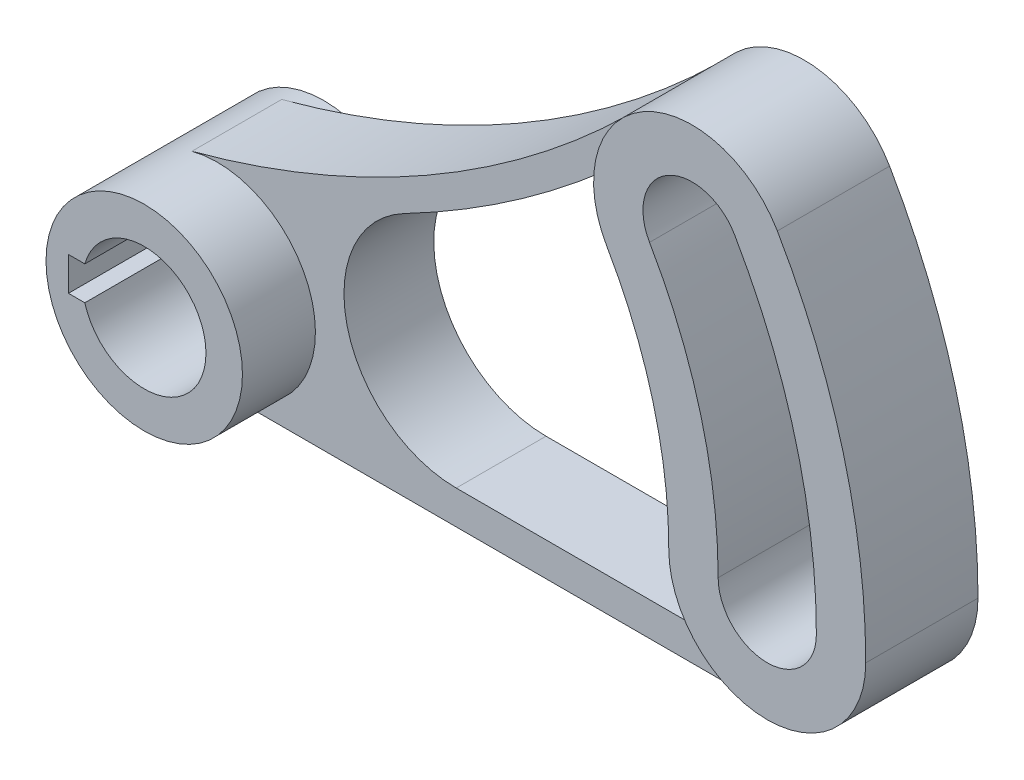
ISO-10303-21;
HEADER;
FILE_DESCRIPTION(('STEP AP214'),'2;1');
FILE_NAME('part.step','',(''),(''),'','','');
FILE_SCHEMA(('AUTOMOTIVE_DESIGN { 1 0 10303 214 1 1 1 1 }'));
ENDSEC;
DATA;
#1=APPLICATION_CONTEXT('core data for automotive mechanical design processes');
#2=APPLICATION_PROTOCOL_DEFINITION('international standard','automotive_design',2000,#1);
#3=PRODUCT_CONTEXT('',#1,'mechanical');
#4=PRODUCT('Part','Part','',(#3));
#5=PRODUCT_RELATED_PRODUCT_CATEGORY('part','',(#4));
#6=PRODUCT_DEFINITION_FORMATION('','',#4);
#7=PRODUCT_DEFINITION_CONTEXT('part definition',#1,'design');
#8=PRODUCT_DEFINITION('design','',#6,#7);
#9=PRODUCT_DEFINITION_SHAPE('','',#8);
#10=(LENGTH_UNIT() NAMED_UNIT(*) SI_UNIT(.MILLI.,.METRE.));
#11=(NAMED_UNIT(*) PLANE_ANGLE_UNIT() SI_UNIT($,.RADIAN.));
#12=(NAMED_UNIT(*) SI_UNIT($,.STERADIAN.) SOLID_ANGLE_UNIT());
#13=UNCERTAINTY_MEASURE_WITH_UNIT(LENGTH_MEASURE(1.E-05),#10,'distance_accuracy_value','');
#14=(GEOMETRIC_REPRESENTATION_CONTEXT(3) GLOBAL_UNCERTAINTY_ASSIGNED_CONTEXT((#13)) GLOBAL_UNIT_ASSIGNED_CONTEXT((#10,
#11,#12)) REPRESENTATION_CONTEXT('',''));
#15=CARTESIAN_POINT('',(0.,0.,0.));
#16=DIRECTION('',(0.,0.,1.));
#17=DIRECTION('',(1.,0.,0.));
#18=AXIS2_PLACEMENT_3D('',#15,#16,#17);
#19=CARTESIAN_POINT('',(0.,0.,0.));
#20=DIRECTION('',(0.,0.,1.));
#21=DIRECTION('',(1.,0.,0.));
#22=AXIS2_PLACEMENT_3D('',#19,#20,#21);
#23=PLANE('',#22);
#24=CARTESIAN_POINT('',(100.,0.,0.));
#25=DIRECTION('',(0.,0.,-1.));
#26=DIRECTION('',(-1.,0.,0.));
#27=AXIS2_PLACEMENT_3D('',#24,#25,#26);
#28=CIRCLE('',#27,17.5454153646748);
#29=CARTESIAN_POINT('',(98.7384135705524,-17.5,0.));
#30=VERTEX_POINT('',#29);
#31=CARTESIAN_POINT('',(86.7489019202571,-11.5,0.));
#32=VERTEX_POINT('',#31);
#33=EDGE_CURVE('E213',#30,#32,#28,.T.);
#34=ORIENTED_EDGE('',*,*,#33,.F.);
#35=DIRECTION('',(1.,0.,0.));
#36=VECTOR('',#35,1.);
#37=CARTESIAN_POINT('',(0.,-17.5,0.));
#38=LINE('',#37,#36);
#39=CARTESIAN_POINT('',(0.,-17.5,0.));
#40=VERTEX_POINT('',#39);
#41=EDGE_CURVE('E292',#40,#30,#38,.T.);
#42=ORIENTED_EDGE('',*,*,#41,.F.);
#43=CARTESIAN_POINT('',(0.,0.,0.));
#44=DIRECTION('',(0.,0.,-1.));
#45=DIRECTION('',(-1.,0.,0.));
#46=AXIS2_PLACEMENT_3D('',#43,#44,#45);
#47=CIRCLE('',#46,17.5);
#48=CARTESIAN_POINT('',(-4.51320791235317,16.9080145002266,0.));
#49=VERTEX_POINT('',#48);
#50=EDGE_CURVE('E267',#49,#40,#47,.T.);
#51=ORIENTED_EDGE('',*,*,#50,.F.);
#52=CARTESIAN_POINT('',(-49.6452870358849,185.988159502493,0.));
#53=DIRECTION('',(0.,0.,1.));
#54=DIRECTION('',(1.,0.,0.));
#55=AXIS2_PLACEMENT_3D('',#52,#53,#54);
#56=CIRCLE('',#55,175.);
#57=CARTESIAN_POINT('',(73.3637035666173,61.5141130873722,0.));
#58=VERTEX_POINT('',#57);
#59=EDGE_CURVE('E310',#49,#58,#56,.T.);
#60=ORIENTED_EDGE('',*,*,#59,.T.);
#61=CARTESIAN_POINT('',(86.6025403784438,50.0000000000001,0.));
#62=DIRECTION('',(0.,0.,-1.));
#63=DIRECTION('',(-1.,0.,0.));
#64=AXIS2_PLACEMENT_3D('',#61,#62,#63);
#65=CIRCLE('',#64,17.5454153646748);
#66=CARTESIAN_POINT('',(69.0694132467358,50.6565464967017,0.));
#67=VERTEX_POINT('',#66);
#68=EDGE_CURVE('E217',#67,#58,#65,.T.);
#69=ORIENTED_EDGE('',*,*,#68,.F.);
#70=CARTESIAN_POINT('',(-49.6452870358849,185.988159502493,0.));
#71=DIRECTION('',(0.,0.,1.));
#72=DIRECTION('',(1.,0.,0.));
#73=AXIS2_PLACEMENT_3D('',#70,#71,#72);
#74=CIRCLE('',#73,180.021736304096);
#75=CARTESIAN_POINT('',(33.3640585971692,26.2468871915654,0.));
#76=VERTEX_POINT('',#75);
#77=EDGE_CURVE('E284',#76,#67,#74,.T.);
#78=ORIENTED_EDGE('',*,*,#77,.F.);
#79=CARTESIAN_POINT('',(42.5862055820014,8.50000000000001,0.));
#80=DIRECTION('',(0.,0.,1.));
#81=DIRECTION('',(1.,0.,0.));
#82=AXIS2_PLACEMENT_3D('',#79,#80,#81);
#83=CIRCLE('',#82,20.);
#84=CARTESIAN_POINT('',(42.5862055820014,-11.5,0.));
#85=VERTEX_POINT('',#84);
#86=EDGE_CURVE('E308',#76,#85,#83,.T.);
#87=ORIENTED_EDGE('',*,*,#86,.T.);
#88=DIRECTION('',(1.,0.,0.));
#89=VECTOR('',#88,1.);
#90=CARTESIAN_POINT('',(0.,-11.5,0.));
#91=LINE('',#90,#89);
#92=EDGE_CURVE('E303',#85,#32,#91,.T.);
#93=ORIENTED_EDGE('',*,*,#92,.T.);
#94=EDGE_LOOP('',(#34,#42,#51,#60,#69,#78,#87,#93));
#95=FACE_BOUND('',#94,.T.);
#96=ADVANCED_FACE('F41',(#95),#23,.F.);
#97=CARTESIAN_POINT('',(0.,0.,16.));
#98=DIRECTION('',(0.,0.,1.));
#99=DIRECTION('',(1.,0.,0.));
#100=AXIS2_PLACEMENT_3D('',#97,#98,#99);
#101=PLANE('',#100);
#102=CARTESIAN_POINT('',(-49.6452870358849,185.988159502493,16.));
#103=DIRECTION('',(0.,0.,1.));
#104=DIRECTION('',(1.,0.,0.));
#105=AXIS2_PLACEMENT_3D('',#102,#103,#104);
#106=CIRCLE('',#105,180.021736304096);
#107=CARTESIAN_POINT('',(33.3640585971692,26.2468871915654,16.));
#108=VERTEX_POINT('',#107);
#109=CARTESIAN_POINT('',(69.0694132467358,50.6565464967017,16.));
#110=VERTEX_POINT('',#109);
#111=EDGE_CURVE('E288',#108,#110,#106,.T.);
#112=ORIENTED_EDGE('',*,*,#111,.T.);
#113=CARTESIAN_POINT('',(86.6025403784438,50.0000000000001,16.));
#114=DIRECTION('',(0.,0.,1.));
#115=DIRECTION('',(1.,0.,0.));
#116=AXIS2_PLACEMENT_3D('',#113,#114,#115);
#117=CIRCLE('',#116,17.5454153646748);
#118=CARTESIAN_POINT('',(73.3637035666185,61.5141130873735,16.));
#119=VERTEX_POINT('',#118);
#120=EDGE_CURVE('E11',#110,#119,#117,.F.);
#121=ORIENTED_EDGE('',*,*,#120,.T.);
#122=CARTESIAN_POINT('',(-49.6452870358849,185.988159502493,16.));
#123=DIRECTION('',(0.,0.,1.));
#124=DIRECTION('',(1.,0.,0.));
#125=AXIS2_PLACEMENT_3D('',#122,#123,#124);
#126=CIRCLE('',#125,175.);
#127=CARTESIAN_POINT('',(-4.51320791235317,16.9080145002266,16.));
#128=VERTEX_POINT('',#127);
#129=EDGE_CURVE('E299',#128,#119,#126,.T.);
#130=ORIENTED_EDGE('',*,*,#129,.F.);
#131=CARTESIAN_POINT('',(0.,0.,16.));
#132=DIRECTION('',(0.,0.,1.));
#133=DIRECTION('',(1.,0.,0.));
#134=AXIS2_PLACEMENT_3D('',#131,#132,#133);
#135=CIRCLE('',#134,17.5);
#136=CARTESIAN_POINT('',(0.,-17.5,16.));
#137=VERTEX_POINT('',#136);
#138=EDGE_CURVE('E282',#137,#128,#135,.T.);
#139=ORIENTED_EDGE('',*,*,#138,.F.);
#140=DIRECTION('',(1.,0.,0.));
#141=VECTOR('',#140,1.);
#142=CARTESIAN_POINT('',(0.,-17.5,16.));
#143=LINE('',#142,#141);
#144=CARTESIAN_POINT('',(98.7384135705524,-17.5,16.));
#145=VERTEX_POINT('',#144);
#146=EDGE_CURVE('E198',#137,#145,#143,.T.);
#147=ORIENTED_EDGE('',*,*,#146,.T.);
#148=CARTESIAN_POINT('',(100.,0.,16.));
#149=DIRECTION('',(0.,0.,1.));
#150=DIRECTION('',(1.,0.,0.));
#151=AXIS2_PLACEMENT_3D('',#148,#149,#150);
#152=CIRCLE('',#151,17.5454153646748);
#153=CARTESIAN_POINT('',(86.7489019202571,-11.5,16.));
#154=VERTEX_POINT('',#153);
#155=EDGE_CURVE('E47',#145,#154,#152,.F.);
#156=ORIENTED_EDGE('',*,*,#155,.T.);
#157=DIRECTION('',(1.,0.,0.));
#158=VECTOR('',#157,1.);
#159=CARTESIAN_POINT('',(0.,-11.5,16.));
#160=LINE('',#159,#158);
#161=CARTESIAN_POINT('',(42.5862055820014,-11.5,16.));
#162=VERTEX_POINT('',#161);
#163=EDGE_CURVE('E289',#162,#154,#160,.T.);
#164=ORIENTED_EDGE('',*,*,#163,.F.);
#165=CARTESIAN_POINT('',(42.5862055820014,8.50000000000001,16.));
#166=DIRECTION('',(0.,0.,1.));
#167=DIRECTION('',(1.,0.,0.));
#168=AXIS2_PLACEMENT_3D('',#165,#166,#167);
#169=CIRCLE('',#168,20.);
#170=EDGE_CURVE('E294',#108,#162,#169,.T.);
#171=ORIENTED_EDGE('',*,*,#170,.F.);
#172=EDGE_LOOP('',(#112,#121,#130,#139,#147,#156,#164,#171));
#173=FACE_BOUND('',#172,.T.);
#174=ADVANCED_FACE('F363',(#173),#101,.T.);
#175=CARTESIAN_POINT('',(0.,0.,29.));
#176=DIRECTION('',(0.,0.,1.));
#177=DIRECTION('',(1.,0.,0.));
#178=AXIS2_PLACEMENT_3D('',#175,#176,#177);
#179=PLANE('',#178);
#180=CARTESIAN_POINT('',(0.,0.,29.));
#181=DIRECTION('',(0.,0.,1.));
#182=DIRECTION('',(1.,0.,0.));
#183=AXIS2_PLACEMENT_3D('',#180,#181,#182);
#184=CIRCLE('',#183,17.5);
#185=CARTESIAN_POINT('',(17.5,0.,29.));
#186=VERTEX_POINT('',#185);
#187=EDGE_CURVE('E279',#186,#186,#184,.T.);
#188=ORIENTED_EDGE('',*,*,#187,.T.);
#189=EDGE_LOOP('',(#188));
#190=FACE_BOUND('',#189,.T.);
#191=CARTESIAN_POINT('',(0.,0.,29.));
#192=DIRECTION('',(0.,0.,1.));
#193=DIRECTION('',(1.,0.,0.));
#194=AXIS2_PLACEMENT_3D('',#191,#192,#193);
#195=CIRCLE('',#194,11.);
#196=CARTESIAN_POINT('',(-10.5830052442584,-3.,29.));
#197=VERTEX_POINT('',#196);
#198=CARTESIAN_POINT('',(-10.5830052442584,3.,29.));
#199=VERTEX_POINT('',#198);
#200=EDGE_CURVE('E260',#197,#199,#195,.T.);
#201=ORIENTED_EDGE('',*,*,#200,.F.);
#202=DIRECTION('',(-1.,0.,0.));
#203=VECTOR('',#202,1.);
#204=CARTESIAN_POINT('',(0.,-3.,29.));
#205=LINE('',#204,#203);
#206=CARTESIAN_POINT('',(-13.5,-3.,29.));
#207=VERTEX_POINT('',#206);
#208=EDGE_CURVE('E65',#197,#207,#205,.T.);
#209=ORIENTED_EDGE('',*,*,#208,.T.);
#210=DIRECTION('',(0.,1.,0.));
#211=VECTOR('',#210,1.);
#212=CARTESIAN_POINT('',(-13.5,0.,29.));
#213=LINE('',#212,#211);
#214=CARTESIAN_POINT('',(-13.5,3.,29.));
#215=VERTEX_POINT('',#214);
#216=EDGE_CURVE('E263',#207,#215,#213,.T.);
#217=ORIENTED_EDGE('',*,*,#216,.T.);
#218=DIRECTION('',(1.,0.,0.));
#219=VECTOR('',#218,1.);
#220=CARTESIAN_POINT('',(0.,3.,29.));
#221=LINE('',#220,#219);
#222=EDGE_CURVE('E257',#215,#199,#221,.T.);
#223=ORIENTED_EDGE('',*,*,#222,.T.);
#224=EDGE_LOOP('',(#201,#209,#217,#223));
#225=FACE_BOUND('',#224,.T.);
#226=ADVANCED_FACE('F413',(#190,#225),#179,.T.);
#227=CARTESIAN_POINT('',(0.,0.,-3.));
#228=DIRECTION('',(0.,0.,-1.));
#229=DIRECTION('',(-1.,0.,0.));
#230=AXIS2_PLACEMENT_3D('',#227,#228,#229);
#231=PLANE('',#230);
#232=CARTESIAN_POINT('',(0.,0.,-3.));
#233=DIRECTION('',(0.,0.,-1.));
#234=DIRECTION('',(-1.,0.,0.));
#235=AXIS2_PLACEMENT_3D('',#232,#233,#234);
#236=CIRCLE('',#235,17.5);
#237=CARTESIAN_POINT('',(-17.5,0.,-3.));
#238=VERTEX_POINT('',#237);
#239=EDGE_CURVE('E274',#238,#238,#236,.T.);
#240=ORIENTED_EDGE('',*,*,#239,.T.);
#241=EDGE_LOOP('',(#240));
#242=FACE_BOUND('',#241,.T.);
#243=DIRECTION('',(0.,-1.,0.));
#244=VECTOR('',#243,1.);
#245=CARTESIAN_POINT('',(-13.5,0.,-3.));
#246=LINE('',#245,#244);
#247=CARTESIAN_POINT('',(-13.5,3.,-3.));
#248=VERTEX_POINT('',#247);
#249=CARTESIAN_POINT('',(-13.5,-3.,-3.));
#250=VERTEX_POINT('',#249);
#251=EDGE_CURVE('E354',#248,#250,#246,.T.);
#252=ORIENTED_EDGE('',*,*,#251,.T.);
#253=DIRECTION('',(1.,0.,0.));
#254=VECTOR('',#253,1.);
#255=CARTESIAN_POINT('',(0.,-3.,-3.));
#256=LINE('',#255,#254);
#257=CARTESIAN_POINT('',(-10.5830052442584,-3.,-3.));
#258=VERTEX_POINT('',#257);
#259=EDGE_CURVE('E351',#250,#258,#256,.T.);
#260=ORIENTED_EDGE('',*,*,#259,.T.);
#261=CARTESIAN_POINT('',(0.,0.,-3.));
#262=DIRECTION('',(0.,0.,-1.));
#263=DIRECTION('',(-1.,0.,0.));
#264=AXIS2_PLACEMENT_3D('',#261,#262,#263);
#265=CIRCLE('',#264,11.);
#266=CARTESIAN_POINT('',(-10.5830052442584,3.,-3.));
#267=VERTEX_POINT('',#266);
#268=EDGE_CURVE('E286',#267,#258,#265,.T.);
#269=ORIENTED_EDGE('',*,*,#268,.F.);
#270=DIRECTION('',(-1.,0.,0.));
#271=VECTOR('',#270,1.);
#272=CARTESIAN_POINT('',(0.,3.,-3.));
#273=LINE('',#272,#271);
#274=EDGE_CURVE('E349',#267,#248,#273,.T.);
#275=ORIENTED_EDGE('',*,*,#274,.T.);
#276=EDGE_LOOP('',(#252,#260,#269,#275));
#277=FACE_BOUND('',#276,.T.);
#278=ADVANCED_FACE('F468',(#242,#277),#231,.T.);
#279=CARTESIAN_POINT('',(86.6025403784438,50.0000000000001,16.));
#280=DIRECTION('',(0.,0.,-1.));
#281=DIRECTION('',(-1.,0.,0.));
#282=AXIS2_PLACEMENT_3D('',#279,#280,#281);
#283=CYLINDRICAL_SURFACE('',#282,17.5454153646748);
#284=ORIENTED_EDGE('',*,*,#68,.T.);
#285=DIRECTION('',(0.,0.,-1.));
#286=VECTOR('',#285,1.);
#287=CARTESIAN_POINT('',(73.3637035666185,61.5141130873735,16.));
#288=LINE('',#287,#286);
#289=EDGE_CURVE('E290',#119,#58,#288,.T.);
#290=ORIENTED_EDGE('',*,*,#289,.F.);
#291=ORIENTED_EDGE('',*,*,#120,.F.);
#292=DIRECTION('',(0.,0.,-1.));
#293=VECTOR('',#292,1.);
#294=CARTESIAN_POINT('',(69.0694132467358,50.6565464967017,16.));
#295=LINE('',#294,#293);
#296=EDGE_CURVE('E320',#110,#67,#295,.T.);
#297=ORIENTED_EDGE('',*,*,#296,.T.);
#298=EDGE_LOOP('',(#284,#290,#291,#297));
#299=FACE_BOUND('',#298,.T.);
#300=DIRECTION('',(0.,0.,-1.));
#301=VECTOR('',#300,1.);
#302=CARTESIAN_POINT('',(101.797315804202,58.7727076823375,16.));
#303=LINE('',#302,#301);
#304=CARTESIAN_POINT('',(101.797315804202,58.7727076823375,18.));
#305=VERTEX_POINT('',#304);
#306=CARTESIAN_POINT('',(101.797315804202,58.7727076823375,-2.));
#307=VERTEX_POINT('',#306);
#308=EDGE_CURVE('E314',#305,#307,#303,.T.);
#309=ORIENTED_EDGE('',*,*,#308,.T.);
#310=CARTESIAN_POINT('',(86.6025403784438,50.0000000000001,-2.));
#311=DIRECTION('',(0.,0.,-1.));
#312=DIRECTION('',(-1.,0.,0.));
#313=AXIS2_PLACEMENT_3D('',#310,#311,#312);
#314=CIRCLE('',#313,17.5454153646748);
#315=CARTESIAN_POINT('',(71.4077649526857,41.2272923176627,-2.));
#316=VERTEX_POINT('',#315);
#317=EDGE_CURVE('E222',#316,#307,#314,.T.);
#318=ORIENTED_EDGE('',*,*,#317,.F.);
#319=DIRECTION('',(0.,0.,-1.));
#320=VECTOR('',#319,1.);
#321=CARTESIAN_POINT('',(71.4077649526856,41.2272923176626,16.));
#322=LINE('',#321,#320);
#323=CARTESIAN_POINT('',(71.4077649526857,41.2272923176627,18.));
#324=VERTEX_POINT('',#323);
#325=EDGE_CURVE('E336',#324,#316,#322,.T.);
#326=ORIENTED_EDGE('',*,*,#325,.F.);
#327=CARTESIAN_POINT('',(86.6025403784438,50.0000000000001,18.));
#328=DIRECTION('',(0.,0.,1.));
#329=DIRECTION('',(1.,0.,0.));
#330=AXIS2_PLACEMENT_3D('',#327,#328,#329);
#331=CIRCLE('',#330,17.5454153646748);
#332=EDGE_CURVE('E244',#305,#324,#331,.T.);
#333=ORIENTED_EDGE('',*,*,#332,.F.);
#334=EDGE_LOOP('',(#309,#318,#326,#333));
#335=FACE_BOUND('',#334,.T.);
#336=ADVANCED_FACE('F385',(#299,#335),#283,.T.);
#337=CARTESIAN_POINT('',(-49.6452870358849,185.988159502493,16.));
#338=DIRECTION('',(0.,0.,-1.));
#339=DIRECTION('',(-1.,0.,0.));
#340=AXIS2_PLACEMENT_3D('',#337,#338,#339);
#341=CYLINDRICAL_SURFACE('',#340,175.);
#342=ORIENTED_EDGE('',*,*,#59,.F.);
#343=DIRECTION('',(0.,0.,-1.));
#344=VECTOR('',#343,1.);
#345=CARTESIAN_POINT('',(-4.51320791235317,16.9080145002266,16.));
#346=LINE('',#345,#344);
#347=EDGE_CURVE('E324',#128,#49,#346,.T.);
#348=ORIENTED_EDGE('',*,*,#347,.F.);
#349=ORIENTED_EDGE('',*,*,#129,.T.);
#350=ORIENTED_EDGE('',*,*,#289,.T.);
#351=EDGE_LOOP('',(#342,#348,#349,#350));
#352=FACE_BOUND('',#351,.T.);
#353=ADVANCED_FACE('F390',(#352),#341,.F.);
#354=CARTESIAN_POINT('',(0.,0.,16.));
#355=DIRECTION('',(0.,0.,-1.));
#356=DIRECTION('',(-1.,0.,0.));
#357=AXIS2_PLACEMENT_3D('',#354,#355,#356);
#358=CYLINDRICAL_SURFACE('',#357,17.5);
#359=ORIENTED_EDGE('',*,*,#347,.T.);
#360=ORIENTED_EDGE('',*,*,#50,.T.);
#361=DIRECTION('',(0.,0.,-1.));
#362=VECTOR('',#361,1.);
#363=CARTESIAN_POINT('',(0.,-17.5,16.));
#364=LINE('',#363,#362);
#365=EDGE_CURVE('E325',#137,#40,#364,.T.);
#366=ORIENTED_EDGE('',*,*,#365,.F.);
#367=ORIENTED_EDGE('',*,*,#138,.T.);
#368=EDGE_LOOP('',(#359,#360,#366,#367));
#369=FACE_BOUND('',#368,.T.);
#370=ORIENTED_EDGE('',*,*,#187,.F.);
#371=EDGE_LOOP('',(#370));
#372=FACE_BOUND('',#371,.T.);
#373=ORIENTED_EDGE('',*,*,#239,.F.);
#374=EDGE_LOOP('',(#373));
#375=FACE_BOUND('',#374,.T.);
#376=ADVANCED_FACE('F388',(#369,#372,#375),#358,.T.);
#377=CARTESIAN_POINT('',(0.,-17.5,16.));
#378=DIRECTION('',(0.,1.,0.));
#379=DIRECTION('',(0.,0.,1.));
#380=AXIS2_PLACEMENT_3D('',#377,#378,#379);
#381=PLANE('',#380);
#382=ORIENTED_EDGE('',*,*,#41,.T.);
#383=DIRECTION('',(-1.,0.,0.));
#384=VECTOR('',#383,1.);
#385=CARTESIAN_POINT('',(0.,-17.5,0.));
#386=LINE('',#385,#384);
#387=CARTESIAN_POINT('',(101.261586429448,-17.5,0.));
#388=VERTEX_POINT('',#387);
#389=EDGE_CURVE('E229',#388,#30,#386,.T.);
#390=ORIENTED_EDGE('',*,*,#389,.F.);
#391=DIRECTION('',(0.,0.,-1.));
#392=VECTOR('',#391,1.);
#393=CARTESIAN_POINT('',(101.261586429448,-17.5,16.));
#394=LINE('',#393,#392);
#395=CARTESIAN_POINT('',(101.261586429448,-17.5,16.));
#396=VERTEX_POINT('',#395);
#397=EDGE_CURVE('E317',#396,#388,#394,.T.);
#398=ORIENTED_EDGE('',*,*,#397,.F.);
#399=EDGE_CURVE('E57',#145,#396,#143,.T.);
#400=ORIENTED_EDGE('',*,*,#399,.F.);
#401=ORIENTED_EDGE('',*,*,#146,.F.);
#402=ORIENTED_EDGE('',*,*,#365,.T.);
#403=EDGE_LOOP('',(#382,#390,#398,#400,#401,#402));
#404=FACE_BOUND('',#403,.T.);
#405=ADVANCED_FACE('F392',(#404),#381,.F.);
#406=CARTESIAN_POINT('',(100.,0.,16.));
#407=DIRECTION('',(0.,0.,-1.));
#408=DIRECTION('',(-1.,0.,0.));
#409=AXIS2_PLACEMENT_3D('',#406,#407,#408);
#410=CYLINDRICAL_SURFACE('',#409,17.5454153646748);
#411=CARTESIAN_POINT('',(100.,0.,-2.));
#412=DIRECTION('',(0.,0.,-1.));
#413=DIRECTION('',(-1.,0.,0.));
#414=AXIS2_PLACEMENT_3D('',#411,#412,#413);
#415=CIRCLE('',#414,17.5454153646748);
#416=CARTESIAN_POINT('',(117.545415364675,0.,-2.));
#417=VERTEX_POINT('',#416);
#418=CARTESIAN_POINT('',(82.4545846353252,0.,-2.));
#419=VERTEX_POINT('',#418);
#420=EDGE_CURVE('E212',#417,#419,#415,.T.);
#421=ORIENTED_EDGE('',*,*,#420,.F.);
#422=DIRECTION('',(0.,0.,-1.));
#423=VECTOR('',#422,1.);
#424=CARTESIAN_POINT('',(117.545415364675,0.,16.));
#425=LINE('',#424,#423);
#426=CARTESIAN_POINT('',(117.545415364675,0.,18.));
#427=VERTEX_POINT('',#426);
#428=EDGE_CURVE('E316',#427,#417,#425,.T.);
#429=ORIENTED_EDGE('',*,*,#428,.F.);
#430=CARTESIAN_POINT('',(100.,0.,18.));
#431=DIRECTION('',(0.,0.,1.));
#432=DIRECTION('',(1.,0.,0.));
#433=AXIS2_PLACEMENT_3D('',#430,#431,#432);
#434=CIRCLE('',#433,17.5454153646748);
#435=CARTESIAN_POINT('',(82.4545846353252,0.,18.));
#436=VERTEX_POINT('',#435);
#437=EDGE_CURVE('E248',#436,#427,#434,.T.);
#438=ORIENTED_EDGE('',*,*,#437,.F.);
#439=DIRECTION('',(0.,0.,-1.));
#440=VECTOR('',#439,1.);
#441=CARTESIAN_POINT('',(82.4545846353252,0.,16.));
#442=LINE('',#441,#440);
#443=EDGE_CURVE('E337',#436,#419,#442,.T.);
#444=ORIENTED_EDGE('',*,*,#443,.T.);
#445=EDGE_LOOP('',(#421,#429,#438,#444));
#446=FACE_BOUND('',#445,.T.);
#447=ORIENTED_EDGE('',*,*,#397,.T.);
#448=EDGE_CURVE('E230',#388,#30,#28,.T.);
#449=ORIENTED_EDGE('',*,*,#448,.T.);
#450=ORIENTED_EDGE('',*,*,#33,.T.);
#451=DIRECTION('',(0.,0.,-1.));
#452=VECTOR('',#451,1.);
#453=CARTESIAN_POINT('',(86.7489019202571,-11.5,16.));
#454=LINE('',#453,#452);
#455=EDGE_CURVE('E333',#154,#32,#454,.T.);
#456=ORIENTED_EDGE('',*,*,#455,.F.);
#457=ORIENTED_EDGE('',*,*,#155,.F.);
#458=CARTESIAN_POINT('',(100.,0.,16.));
#459=DIRECTION('',(0.,0.,1.));
#460=DIRECTION('',(1.,0.,0.));
#461=AXIS2_PLACEMENT_3D('',#458,#459,#460);
#462=CIRCLE('',#461,17.5454153646748);
#463=EDGE_CURVE('E243',#145,#396,#462,.T.);
#464=ORIENTED_EDGE('',*,*,#463,.T.);
#465=EDGE_LOOP('',(#447,#449,#450,#456,#457,#464));
#466=FACE_BOUND('',#465,.T.);
#467=ADVANCED_FACE('F364',(#446,#466),#410,.T.);
#468=CARTESIAN_POINT('',(-49.6452870358849,185.988159502493,16.));
#469=DIRECTION('',(0.,0.,-1.));
#470=DIRECTION('',(-1.,0.,0.));
#471=AXIS2_PLACEMENT_3D('',#468,#469,#470);
#472=CYLINDRICAL_SURFACE('',#471,180.021736304096);
#473=ORIENTED_EDGE('',*,*,#77,.T.);
#474=ORIENTED_EDGE('',*,*,#296,.F.);
#475=ORIENTED_EDGE('',*,*,#111,.F.);
#476=DIRECTION('',(0.,0.,-1.));
#477=VECTOR('',#476,1.);
#478=CARTESIAN_POINT('',(33.3640585971692,26.2468871915654,16.));
#479=LINE('',#478,#477);
#480=EDGE_CURVE('E329',#108,#76,#479,.T.);
#481=ORIENTED_EDGE('',*,*,#480,.T.);
#482=EDGE_LOOP('',(#473,#474,#475,#481));
#483=FACE_BOUND('',#482,.T.);
#484=ADVANCED_FACE('F377',(#483),#472,.T.);
#485=CARTESIAN_POINT('',(0.,0.,16.));
#486=DIRECTION('',(0.,0.,-1.));
#487=DIRECTION('',(-1.,0.,0.));
#488=AXIS2_PLACEMENT_3D('',#485,#486,#487);
#489=CYLINDRICAL_SURFACE('',#488,82.4545846353252);
#490=ORIENTED_EDGE('',*,*,#325,.T.);
#491=CARTESIAN_POINT('',(0.,0.,-2.));
#492=DIRECTION('',(0.,0.,1.));
#493=DIRECTION('',(-1.,0.,0.));
#494=AXIS2_PLACEMENT_3D('',#491,#492,#493);
#495=CIRCLE('',#494,82.4545846353252);
#496=EDGE_CURVE('E220',#419,#316,#495,.T.);
#497=ORIENTED_EDGE('',*,*,#496,.F.);
#498=ORIENTED_EDGE('',*,*,#443,.F.);
#499=CARTESIAN_POINT('',(0.,0.,18.));
#500=DIRECTION('',(0.,0.,-1.));
#501=DIRECTION('',(1.,0.,0.));
#502=AXIS2_PLACEMENT_3D('',#499,#500,#501);
#503=CIRCLE('',#502,82.4545846353252);
#504=EDGE_CURVE('E241',#324,#436,#503,.T.);
#505=ORIENTED_EDGE('',*,*,#504,.F.);
#506=EDGE_LOOP('',(#490,#497,#498,#505));
#507=FACE_BOUND('',#506,.T.);
#508=ADVANCED_FACE('F437',(#507),#489,.F.);
#509=CARTESIAN_POINT('',(0.,-11.5,16.));
#510=DIRECTION('',(0.,1.,0.));
#511=DIRECTION('',(-1.,0.,0.));
#512=AXIS2_PLACEMENT_3D('',#509,#510,#511);
#513=PLANE('',#512);
#514=ORIENTED_EDGE('',*,*,#92,.F.);
#515=DIRECTION('',(0.,0.,-1.));
#516=VECTOR('',#515,1.);
#517=CARTESIAN_POINT('',(42.5862055820014,-11.5,16.));
#518=LINE('',#517,#516);
#519=EDGE_CURVE('E335',#162,#85,#518,.T.);
#520=ORIENTED_EDGE('',*,*,#519,.F.);
#521=ORIENTED_EDGE('',*,*,#163,.T.);
#522=ORIENTED_EDGE('',*,*,#455,.T.);
#523=EDGE_LOOP('',(#514,#520,#521,#522));
#524=FACE_BOUND('',#523,.T.);
#525=ADVANCED_FACE('F367',(#524),#513,.T.);
#526=CARTESIAN_POINT('',(0.,0.,16.));
#527=DIRECTION('',(0.,0.,-1.));
#528=DIRECTION('',(-1.,0.,0.));
#529=AXIS2_PLACEMENT_3D('',#526,#527,#528);
#530=CYLINDRICAL_SURFACE('',#529,91.25);
#531=DIRECTION('',(0.,0.,-1.));
#532=VECTOR('',#531,1.);
#533=CARTESIAN_POINT('',(91.2500000000001,0.,16.));
#534=LINE('',#533,#532);
#535=CARTESIAN_POINT('',(91.25,0.,18.));
#536=VERTEX_POINT('',#535);
#537=CARTESIAN_POINT('',(91.25,0.,-2.));
#538=VERTEX_POINT('',#537);
#539=EDGE_CURVE('E183',#536,#538,#534,.T.);
#540=ORIENTED_EDGE('',*,*,#539,.T.);
#541=CARTESIAN_POINT('',(0.,0.,-2.));
#542=DIRECTION('',(0.,0.,1.));
#543=DIRECTION('',(-1.,0.,0.));
#544=AXIS2_PLACEMENT_3D('',#541,#542,#543);
#545=CIRCLE('',#544,91.25);
#546=CARTESIAN_POINT('',(79.02481809533,45.6250000000001,-2.));
#547=VERTEX_POINT('',#546);
#548=EDGE_CURVE('E187',#538,#547,#545,.T.);
#549=ORIENTED_EDGE('',*,*,#548,.T.);
#550=DIRECTION('',(0.,0.,-1.));
#551=VECTOR('',#550,1.);
#552=CARTESIAN_POINT('',(79.02481809533,45.6250000000001,16.));
#553=LINE('',#552,#551);
#554=CARTESIAN_POINT('',(79.02481809533,45.6250000000001,18.));
#555=VERTEX_POINT('',#554);
#556=EDGE_CURVE('E334',#555,#547,#553,.T.);
#557=ORIENTED_EDGE('',*,*,#556,.F.);
#558=CARTESIAN_POINT('',(0.,0.,18.));
#559=DIRECTION('',(0.,0.,-1.));
#560=DIRECTION('',(1.,0.,0.));
#561=AXIS2_PLACEMENT_3D('',#558,#559,#560);
#562=CIRCLE('',#561,91.25);
#563=EDGE_CURVE('E191',#555,#536,#562,.T.);
#564=ORIENTED_EDGE('',*,*,#563,.T.);
#565=EDGE_LOOP('',(#540,#549,#557,#564));
#566=FACE_BOUND('',#565,.T.);
#567=ADVANCED_FACE('F43',(#566),#530,.T.);
#568=CARTESIAN_POINT('',(86.6025403784438,50.0000000000001,16.));
#569=DIRECTION('',(0.,0.,-1.));
#570=DIRECTION('',(-1.,0.,0.));
#571=AXIS2_PLACEMENT_3D('',#568,#569,#570);
#572=CYLINDRICAL_SURFACE('',#571,8.75);
#573=ORIENTED_EDGE('',*,*,#556,.T.);
#574=CARTESIAN_POINT('',(86.6025403784438,50.0000000000001,-2.));
#575=DIRECTION('',(0.,0.,-1.));
#576=DIRECTION('',(-1.,0.,0.));
#577=AXIS2_PLACEMENT_3D('',#574,#575,#576);
#578=CIRCLE('',#577,8.74999999999999);
#579=CARTESIAN_POINT('',(94.1802626615576,54.3750000000001,-2.));
#580=VERTEX_POINT('',#579);
#581=EDGE_CURVE('E210',#547,#580,#578,.T.);
#582=ORIENTED_EDGE('',*,*,#581,.T.);
#583=DIRECTION('',(0.,0.,-1.));
#584=VECTOR('',#583,1.);
#585=CARTESIAN_POINT('',(94.1802626615576,54.3750000000001,16.));
#586=LINE('',#585,#584);
#587=CARTESIAN_POINT('',(94.1802626615576,54.3750000000001,18.));
#588=VERTEX_POINT('',#587);
#589=EDGE_CURVE('E344',#588,#580,#586,.T.);
#590=ORIENTED_EDGE('',*,*,#589,.F.);
#591=CARTESIAN_POINT('',(86.6025403784438,50.0000000000001,18.));
#592=DIRECTION('',(0.,0.,1.));
#593=DIRECTION('',(1.,0.,0.));
#594=AXIS2_PLACEMENT_3D('',#591,#592,#593);
#595=CIRCLE('',#594,8.74999999999999);
#596=EDGE_CURVE('E235',#588,#555,#595,.T.);
#597=ORIENTED_EDGE('',*,*,#596,.T.);
#598=EDGE_LOOP('',(#573,#582,#590,#597));
#599=FACE_BOUND('',#598,.T.);
#600=ADVANCED_FACE('F451',(#599),#572,.F.);
#601=CARTESIAN_POINT('',(0.,0.,16.));
#602=DIRECTION('',(0.,0.,-1.));
#603=DIRECTION('',(-1.,0.,0.));
#604=AXIS2_PLACEMENT_3D('',#601,#602,#603);
#605=CYLINDRICAL_SURFACE('',#604,108.75);
#606=ORIENTED_EDGE('',*,*,#589,.T.);
#607=CARTESIAN_POINT('',(0.,0.,-2.));
#608=DIRECTION('',(0.,0.,-1.));
#609=DIRECTION('',(-1.,0.,0.));
#610=AXIS2_PLACEMENT_3D('',#607,#608,#609);
#611=CIRCLE('',#610,108.75);
#612=CARTESIAN_POINT('',(108.75,0.,-2.));
#613=VERTEX_POINT('',#612);
#614=EDGE_CURVE('E207',#580,#613,#611,.T.);
#615=ORIENTED_EDGE('',*,*,#614,.T.);
#616=DIRECTION('',(0.,0.,-1.));
#617=VECTOR('',#616,1.);
#618=CARTESIAN_POINT('',(108.75,0.,16.));
#619=LINE('',#618,#617);
#620=CARTESIAN_POINT('',(108.75,0.,18.));
#621=VERTEX_POINT('',#620);
#622=EDGE_CURVE('E194',#621,#613,#619,.T.);
#623=ORIENTED_EDGE('',*,*,#622,.F.);
#624=CARTESIAN_POINT('',(0.,0.,18.));
#625=DIRECTION('',(0.,0.,1.));
#626=DIRECTION('',(1.,0.,0.));
#627=AXIS2_PLACEMENT_3D('',#624,#625,#626);
#628=CIRCLE('',#627,108.75);
#629=EDGE_CURVE('E236',#621,#588,#628,.T.);
#630=ORIENTED_EDGE('',*,*,#629,.T.);
#631=EDGE_LOOP('',(#606,#615,#623,#630));
#632=FACE_BOUND('',#631,.T.);
#633=ADVANCED_FACE('F450',(#632),#605,.F.);
#634=CARTESIAN_POINT('',(42.5862055820014,8.50000000000001,16.));
#635=DIRECTION('',(0.,0.,-1.));
#636=DIRECTION('',(-1.,0.,0.));
#637=AXIS2_PLACEMENT_3D('',#634,#635,#636);
#638=CYLINDRICAL_SURFACE('',#637,20.);
#639=ORIENTED_EDGE('',*,*,#86,.F.);
#640=ORIENTED_EDGE('',*,*,#480,.F.);
#641=ORIENTED_EDGE('',*,*,#170,.T.);
#642=ORIENTED_EDGE('',*,*,#519,.T.);
#643=EDGE_LOOP('',(#639,#640,#641,#642));
#644=FACE_BOUND('',#643,.T.);
#645=ADVANCED_FACE('F373',(#644),#638,.F.);
#646=CARTESIAN_POINT('',(100.,0.,16.));
#647=DIRECTION('',(0.,0.,-1.));
#648=DIRECTION('',(-1.,0.,0.));
#649=AXIS2_PLACEMENT_3D('',#646,#647,#648);
#650=CYLINDRICAL_SURFACE('',#649,8.74999999999998);
#651=ORIENTED_EDGE('',*,*,#622,.T.);
#652=CARTESIAN_POINT('',(100.,0.,-2.));
#653=DIRECTION('',(0.,0.,-1.));
#654=DIRECTION('',(-1.,0.,0.));
#655=AXIS2_PLACEMENT_3D('',#652,#653,#654);
#656=CIRCLE('',#655,8.74999999999998);
#657=EDGE_CURVE('E200',#613,#538,#656,.T.);
#658=ORIENTED_EDGE('',*,*,#657,.T.);
#659=ORIENTED_EDGE('',*,*,#539,.F.);
#660=CARTESIAN_POINT('',(100.,0.,18.));
#661=DIRECTION('',(0.,0.,1.));
#662=DIRECTION('',(1.,0.,0.));
#663=AXIS2_PLACEMENT_3D('',#660,#661,#662);
#664=CIRCLE('',#663,8.74999999999998);
#665=EDGE_CURVE('E237',#536,#621,#664,.T.);
#666=ORIENTED_EDGE('',*,*,#665,.T.);
#667=EDGE_LOOP('',(#651,#658,#659,#666));
#668=FACE_BOUND('',#667,.T.);
#669=ADVANCED_FACE('F199',(#668),#650,.F.);
#670=CARTESIAN_POINT('',(0.,0.,16.));
#671=DIRECTION('',(0.,0.,-1.));
#672=DIRECTION('',(-1.,0.,0.));
#673=AXIS2_PLACEMENT_3D('',#670,#671,#672);
#674=CYLINDRICAL_SURFACE('',#673,117.545415364675);
#675=ORIENTED_EDGE('',*,*,#428,.T.);
#676=CARTESIAN_POINT('',(0.,0.,-2.));
#677=DIRECTION('',(0.,0.,-1.));
#678=DIRECTION('',(-1.,0.,0.));
#679=AXIS2_PLACEMENT_3D('',#676,#677,#678);
#680=CIRCLE('',#679,117.545415364675);
#681=EDGE_CURVE('E221',#307,#417,#680,.T.);
#682=ORIENTED_EDGE('',*,*,#681,.F.);
#683=ORIENTED_EDGE('',*,*,#308,.F.);
#684=CARTESIAN_POINT('',(0.,0.,18.));
#685=DIRECTION('',(0.,0.,1.));
#686=DIRECTION('',(1.,0.,0.));
#687=AXIS2_PLACEMENT_3D('',#684,#685,#686);
#688=CIRCLE('',#687,117.545415364675);
#689=EDGE_CURVE('E253',#427,#305,#688,.T.);
#690=ORIENTED_EDGE('',*,*,#689,.F.);
#691=EDGE_LOOP('',(#675,#682,#683,#690));
#692=FACE_BOUND('',#691,.T.);
#693=ADVANCED_FACE('F417',(#692),#674,.T.);
#694=CARTESIAN_POINT('',(0.,-3.,-31.));
#695=DIRECTION('',(0.,1.,0.));
#696=DIRECTION('',(0.,0.,1.));
#697=AXIS2_PLACEMENT_3D('',#694,#695,#696);
#698=PLANE('',#697);
#699=DIRECTION('',(0.,0.,1.));
#700=VECTOR('',#699,1.);
#701=CARTESIAN_POINT('',(-13.5,-3.,-31.));
#702=LINE('',#701,#700);
#703=EDGE_CURVE('E270',#250,#207,#702,.T.);
#704=ORIENTED_EDGE('',*,*,#703,.T.);
#705=ORIENTED_EDGE('',*,*,#208,.F.);
#706=DIRECTION('',(0.,0.,1.));
#707=VECTOR('',#706,1.);
#708=CARTESIAN_POINT('',(-10.5830052442584,-3.,-31.));
#709=LINE('',#708,#707);
#710=EDGE_CURVE('E266',#258,#197,#709,.T.);
#711=ORIENTED_EDGE('',*,*,#710,.F.);
#712=ORIENTED_EDGE('',*,*,#259,.F.);
#713=EDGE_LOOP('',(#704,#705,#711,#712));
#714=FACE_BOUND('',#713,.T.);
#715=ADVANCED_FACE('F420',(#714),#698,.T.);
#716=CARTESIAN_POINT('',(-13.5,0.,-31.));
#717=DIRECTION('',(1.,0.,0.));
#718=DIRECTION('',(0.,0.,-1.));
#719=AXIS2_PLACEMENT_3D('',#716,#717,#718);
#720=PLANE('',#719);
#721=DIRECTION('',(0.,0.,1.));
#722=VECTOR('',#721,1.);
#723=CARTESIAN_POINT('',(-13.5,3.,-31.));
#724=LINE('',#723,#722);
#725=EDGE_CURVE('E269',#248,#215,#724,.T.);
#726=ORIENTED_EDGE('',*,*,#725,.T.);
#727=ORIENTED_EDGE('',*,*,#216,.F.);
#728=ORIENTED_EDGE('',*,*,#703,.F.);
#729=ORIENTED_EDGE('',*,*,#251,.F.);
#730=EDGE_LOOP('',(#726,#727,#728,#729));
#731=FACE_BOUND('',#730,.T.);
#732=ADVANCED_FACE('F426',(#731),#720,.T.);
#733=CARTESIAN_POINT('',(0.,3.,-31.));
#734=DIRECTION('',(0.,-1.,0.));
#735=DIRECTION('',(0.,0.,-1.));
#736=AXIS2_PLACEMENT_3D('',#733,#734,#735);
#737=PLANE('',#736);
#738=DIRECTION('',(0.,0.,1.));
#739=VECTOR('',#738,1.);
#740=CARTESIAN_POINT('',(-10.5830052442584,3.,-31.));
#741=LINE('',#740,#739);
#742=EDGE_CURVE('E275',#267,#199,#741,.T.);
#743=ORIENTED_EDGE('',*,*,#742,.T.);
#744=ORIENTED_EDGE('',*,*,#222,.F.);
#745=ORIENTED_EDGE('',*,*,#725,.F.);
#746=ORIENTED_EDGE('',*,*,#274,.F.);
#747=EDGE_LOOP('',(#743,#744,#745,#746));
#748=FACE_BOUND('',#747,.T.);
#749=ADVANCED_FACE('F562',(#748),#737,.T.);
#750=CARTESIAN_POINT('',(0.,0.,-31.));
#751=DIRECTION('',(0.,0.,1.));
#752=DIRECTION('',(1.,0.,0.));
#753=AXIS2_PLACEMENT_3D('',#750,#751,#752);
#754=CYLINDRICAL_SURFACE('',#753,11.);
#755=ORIENTED_EDGE('',*,*,#268,.T.);
#756=ORIENTED_EDGE('',*,*,#710,.T.);
#757=ORIENTED_EDGE('',*,*,#200,.T.);
#758=ORIENTED_EDGE('',*,*,#742,.F.);
#759=EDGE_LOOP('',(#755,#756,#757,#758));
#760=FACE_BOUND('',#759,.T.);
#761=ADVANCED_FACE('F556',(#760),#754,.F.);
#762=CARTESIAN_POINT('',(43.3012701892219,25.0000000000001,16.));
#763=DIRECTION('',(0.,0.,1.));
#764=DIRECTION('',(1.,0.,0.));
#765=AXIS2_PLACEMENT_3D('',#762,#763,#764);
#766=PLANE('',#765);
#767=ORIENTED_EDGE('',*,*,#463,.F.);
#768=ORIENTED_EDGE('',*,*,#399,.T.);
#769=EDGE_LOOP('',(#767,#768));
#770=FACE_BOUND('',#769,.T.);
#771=ADVANCED_FACE('F441',(#770),#766,.F.);
#772=CARTESIAN_POINT('',(43.3012701892219,25.0000000000001,18.));
#773=DIRECTION('',(0.,0.,1.));
#774=DIRECTION('',(1.,0.,0.));
#775=AXIS2_PLACEMENT_3D('',#772,#773,#774);
#776=PLANE('',#775);
#777=ORIENTED_EDGE('',*,*,#332,.T.);
#778=ORIENTED_EDGE('',*,*,#504,.T.);
#779=ORIENTED_EDGE('',*,*,#437,.T.);
#780=ORIENTED_EDGE('',*,*,#689,.T.);
#781=EDGE_LOOP('',(#777,#778,#779,#780));
#782=FACE_BOUND('',#781,.T.);
#783=ORIENTED_EDGE('',*,*,#563,.F.);
#784=ORIENTED_EDGE('',*,*,#596,.F.);
#785=ORIENTED_EDGE('',*,*,#629,.F.);
#786=ORIENTED_EDGE('',*,*,#665,.F.);
#787=EDGE_LOOP('',(#783,#784,#785,#786));
#788=FACE_BOUND('',#787,.T.);
#789=ADVANCED_FACE('F442',(#782,#788),#776,.T.);
#790=CARTESIAN_POINT('',(50.,0.,0.));
#791=DIRECTION('',(0.,0.,-1.));
#792=DIRECTION('',(-1.,0.,0.));
#793=AXIS2_PLACEMENT_3D('',#790,#791,#792);
#794=PLANE('',#793);
#795=ORIENTED_EDGE('',*,*,#448,.F.);
#796=ORIENTED_EDGE('',*,*,#389,.T.);
#797=EDGE_LOOP('',(#795,#796));
#798=FACE_BOUND('',#797,.T.);
#799=ADVANCED_FACE('F444',(#798),#794,.F.);
#800=CARTESIAN_POINT('',(50.,0.,-2.));
#801=DIRECTION('',(0.,0.,-1.));
#802=DIRECTION('',(-1.,0.,0.));
#803=AXIS2_PLACEMENT_3D('',#800,#801,#802);
#804=PLANE('',#803);
#805=ORIENTED_EDGE('',*,*,#420,.T.);
#806=ORIENTED_EDGE('',*,*,#496,.T.);
#807=ORIENTED_EDGE('',*,*,#317,.T.);
#808=ORIENTED_EDGE('',*,*,#681,.T.);
#809=EDGE_LOOP('',(#805,#806,#807,#808));
#810=FACE_BOUND('',#809,.T.);
#811=ORIENTED_EDGE('',*,*,#548,.F.);
#812=ORIENTED_EDGE('',*,*,#657,.F.);
#813=ORIENTED_EDGE('',*,*,#614,.F.);
#814=ORIENTED_EDGE('',*,*,#581,.F.);
#815=EDGE_LOOP('',(#811,#812,#813,#814));
#816=FACE_BOUND('',#815,.T.);
#817=ADVANCED_FACE('F202',(#810,#816),#804,.T.);
#818=CLOSED_SHELL('',(#96,#174,#226,#278,#336,#353,#376,#405,#467,#484,#508,#525,#567,#600,#633,
#645,#669,#693,#715,#732,#749,#761,#771,#789,#799,#817));
#819=MANIFOLD_SOLID_BREP('B2',#818);
#820=ADVANCED_BREP_SHAPE_REPRESENTATION('',(#18,#819),#14);
#821=SHAPE_DEFINITION_REPRESENTATION(#9,#820);
ENDSEC;
END-ISO-10303-21;
